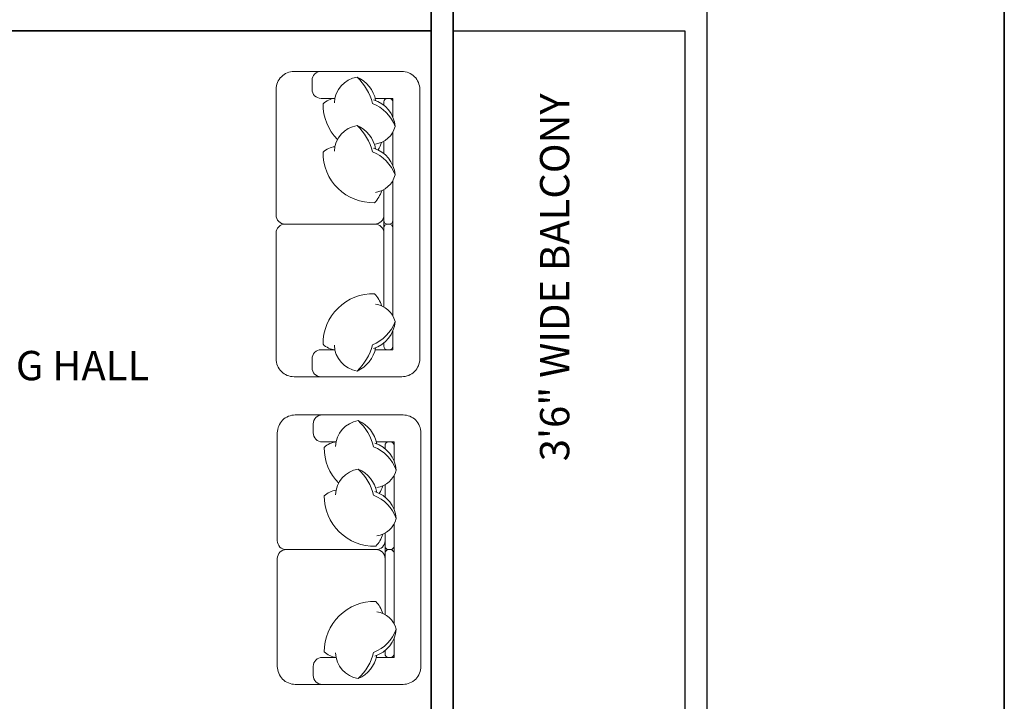
# Model space of a CAD drawing. Units: inches. Extents: x 1088 to 1703, y 668 to 1875.
# Tile 5 of 45: x 1502 to 1703, y 1189 to 1329. Entities that reach past the tile are written whole.
import ezdxf

# ---------------------------------------------------------------- set-up
doc = ezdxf.new("R2010")
doc.units = ezdxf.units.IN
for name, color, linetype, lineweight in [('A-ANNO-DIMS', 2, 'Continuous', 18), ('A-ANNO-TTLB', 7, 'Continuous', 35), ('A-AREA-IDEN', 7, 'Continuous', 18), ('A-FLOR-HRAL', 7, 'Continuous', 25), ('A-FURN', 8, 'Continuous', 13), ('A-WALL', 7, 'Continuous', 35)]:
    doc.layers.add(name, color=color, linetype=linetype, lineweight=lineweight)
doc.styles.get("Standard").update_dxf_attribs({"font": 'arial.ttf'})
doc.dimstyles.get("Standard").update_dxf_attribs({"dimtxt": 0.18, "dimasz": 0.18, "dimexe": 0.18, "dimexo": 0.0625, "dimgap": 0.09, "dimtad": 0, "dimtih": 1, "dimtoh": 1, "dimdec": 4, "dimzin": 0, "dimdsep": 46, "dimtxsty": 'Standard', "dimcen": 0.09, "dimadec": 0, "dimazin": 0, "dimtfac": 1, "dimtdec": 4, "dimtofl": 0, "dimtmove": 0, "dimatfit": 3, "dimfxl": 1, "dimtolj": 1, "dimtzin": 0, "dimarcsym": 0})

# ---------------------------------------------------------------- blocks, each defined once
blk = doc.blocks.new('*D31')
at = {"layer": 'A-ANNO-DIMS', "color": 0, "lineweight": -2, "transparency": 16777216}
for p, q in [((1435.84, 1326.5), (1435.84, 725.55)), ((1585.84, 1326.5), (1585.84, 725.55)), ((1436.02, 725.73), (1510.56, 725.73)), ((1585.66, 725.73), (1511.12, 725.73))]:
    blk.add_line(p, q, dxfattribs=at)
at = {"layer": 'A-ANNO-DIMS', "color": 0, "transparency": 16777216}
for points in [[(1436.02, 725.76), (1436.02, 725.7), (1435.84, 725.73)], [(1585.66, 725.76), (1585.66, 725.7), (1585.84, 725.73)]]:
    blk.add_solid(points, dxfattribs=at)
at = {"layer": 'Defpoints', "color": 0, "transparency": 16777216}
for p in [(1435.84, 1326.56), (1585.84, 1326.56), (1585.84, 725.73)]:
    blk.add_point(p, dxfattribs=at)
at = {"layer": 'A-ANNO-DIMS', "color": 0, "transparency": 16777216, "insert": (1510.84, 725.73), "char_height": 0.18, "attachment_point": 5}
blk.add_mtext('\\A1;150', dxfattribs=at)

msp = doc.modelspace()

# ---------------------------------------------------------------- linework, layer by layer
at = {"layer": 'A-ANNO-TTLB'}
msp.add_lwpolyline([(1088.369, 1874.677), (1703.181, 1874.677), (1703.181, 667.947), (1088.369, 667.947)], close=True, dxfattribs=at)
at = {"layer": 'A-FLOR-HRAL'}
for p, q in [((1642.243, 1331.058), (1642.243, 1181.058)), ((1590.345, 1326.558), (1637.743, 1326.558)), ((1637.743, 1326.558), (1637.743, 1185.558))]:
    msp.add_line(p, q, dxfattribs=at)
at = {"layer": 'A-FURN', "ltscale": 0.03}
for points in [[(1554.082, 1285.137, -0.4142136), (1555.92, 1286.975, -0.4142136), (1554.082, 1288.814), (1554.082, 1314.548, -0.4142136), (1557.759, 1318.225), (1579.817, 1318.225, -0.4142136), (1583.494, 1314.548), (1583.494, 1259.402, -0.4142136), (1579.817, 1255.726), (1557.759, 1255.726, -0.4142136), (1554.082, 1259.402), (1554.082, 1285.137, -0.4142136), (1555.92, 1286.975, -0.4142136), (1554.082, 1288.814)], [(1554.329, 1218.501, -0.4142136), (1556.167, 1220.339, -0.4142136), (1554.329, 1222.178), (1554.329, 1244.236, -0.4142136), (1558.006, 1247.912), (1580.064, 1247.912, -0.4142136), (1583.741, 1244.236), (1583.741, 1196.443, -0.4142136), (1580.064, 1192.766), (1558.006, 1192.766, -0.4142136), (1554.329, 1196.443), (1554.329, 1218.501, -0.4142136), (1556.167, 1220.339, -0.4142136), (1554.329, 1222.178)]]:
    msp.add_lwpolyline(points, format="xyb", dxfattribs=at)
at = {"layer": 'A-FURN'}
for points in [[(1566.121, 1312.71), (1563.273, 1312.71, -0.4142136), (1561.435, 1314.548), (1561.435, 1316.387, -0.4142136), (1563.273, 1318.225)], [(1566.01, 1311.788, -0.3567724), (1570.644, 1317.055, -0.2495421), (1574.462, 1312.282, 9.6168803)], [(1570.644, 1317.055, -0.1477299), (1573.803, 1311.682, -0.2133428), (1578.436, 1306.942, -0.1786618)], [(1566.122, 1312.714, 0.1655406), (1563.693, 1311.577, 0.2002311), (1566.651, 1304.28, 0.1215233)], [(1577.979, 1308.843), (1577.979, 1312.71), (1574.366, 1312.71, -0.4142136)], [(1576.141, 1311.307), (1576.141, 1311.975, -0.4142136), (1576.876, 1312.71), (1577.244, 1312.71, -0.4142136), (1577.979, 1311.975)], [(1574.054, 1312.425, -0.3066635), (1578.436, 1306.942, -0.30633), (1574.435, 1303.36, 0.8728472)], [(1577.979, 1311.975), (1577.979, 1308.843, -0.4142136)], [(1566.01, 1301.885, -0.3567724), (1570.644, 1307.153, -0.2495421), (1574.462, 1302.38, 9.6168803)], [(1570.644, 1307.153, -0.1477299), (1573.803, 1301.78, -0.2133428), (1578.436, 1297.04, -0.1786618)], [(1577.979, 1305.785), (1577.979, 1298.941, -0.4142136)], [(1566.122, 1302.812, 0.1655406), (1563.693, 1301.675, 0.4259892), (1574.224, 1291.351, 0.1215233), (1575.675, 1293.802, -7.1154643)], [(1574.054, 1302.522, -0.3066635), (1578.436, 1297.04, -0.30633), (1574.435, 1293.458, 0.8728472)], [(1574.957, 1302.163, 0.0718654), (1575.675, 1303.704, -7.1154643)], [(1576.141, 1301.405), (1576.141, 1303.934, -0.4142136)], [(1577.979, 1295.883), (1577.979, 1287.711, -0.4142136), (1577.244, 1286.975), (1576.876, 1286.975, -0.4142136), (1576.141, 1287.711), (1576.141, 1294.032, -0.4142136)], [(1576.141, 1288.814, -0.4142136), (1574.303, 1286.975), (1555.92, 1286.975, -0.4142136)], [(1576.141, 1288.814, -0.4142136), (1574.303, 1286.975)], [(1576.141, 1285.137, 0.4142136), (1574.303, 1286.975), (1555.92, 1286.975, 0.4142136)], [(1576.141, 1285.137, 0.4142136), (1574.303, 1286.975)], [(1577.979, 1268.166), (1577.979, 1286.24, 0.4142136), (1577.244, 1286.975), (1576.876, 1286.975, 0.4142136), (1576.141, 1286.24), (1576.141, 1270.017, 0.4142136)], [(1566.122, 1261.236, -0.1655406), (1563.693, 1262.374, -0.4259892), (1574.224, 1272.697, -0.1215233), (1575.675, 1270.247, 7.1154643)], [(1574.054, 1261.526, 0.3066635), (1578.436, 1267.009, 0.30633), (1574.435, 1270.59, -0.8728472)], [(1570.644, 1256.896, 0.1477299), (1573.803, 1262.268, 0.2133428), (1578.436, 1267.009, 0.1786618)], [(1577.979, 1261.976), (1577.979, 1265.108, 0.4142136)], [(1566.01, 1262.163, 0.3567724), (1570.644, 1256.896, 0.2495421), (1574.462, 1261.668, -9.6168803)], [(1576.141, 1262.643), (1576.141, 1261.976, 0.4142136), (1576.876, 1261.24), (1577.244, 1261.24, 0.4142136), (1577.979, 1261.976)], [(1563.273, 1255.726, -0.4142136), (1561.435, 1257.564), (1561.435, 1259.402, -0.4142136), (1563.273, 1261.24), (1566.121, 1261.24)], [(1566.368, 1242.398), (1563.52, 1242.398, -0.4142136), (1561.682, 1244.236), (1561.682, 1246.074, -0.4142136), (1563.52, 1247.912)], [(1566.257, 1241.475, -0.3567724), (1570.89, 1246.743, -0.2495421), (1574.709, 1241.97, 9.6168803)], [(1570.89, 1246.743, -0.1477299), (1574.05, 1241.37, -0.2133428), (1578.683, 1236.63, -0.1786618)], [(1566.369, 1242.402, 0.1655406), (1563.94, 1241.265, 0.2002311), (1566.898, 1233.968, 0.1215233)], [(1574.301, 1242.112, -0.3066635), (1578.683, 1236.63, -0.30633), (1574.681, 1233.048, 0.8728472)], [(1578.226, 1238.531), (1578.226, 1242.398), (1574.613, 1242.398, -0.4142136)], [(1576.388, 1240.995), (1576.388, 1241.663, -0.4142136), (1577.123, 1242.398), (1577.491, 1242.398, -0.4142136), (1578.226, 1241.663)], [(1578.226, 1241.663), (1578.226, 1238.531, -0.4142136)], [(1566.257, 1231.573, -0.3567724), (1570.89, 1236.84, -0.2495421), (1574.709, 1232.068, 9.6168803)], [(1570.89, 1236.84, -0.1477299), (1574.05, 1231.468, -0.2133428), (1578.683, 1226.727, -0.1786618)], [(1578.226, 1235.473), (1578.226, 1228.628, -0.4142136)], [(1566.369, 1232.5, 0.1655406), (1563.94, 1231.362, 0.4259892), (1574.471, 1221.039, 0.1215233), (1575.922, 1223.489, -7.1154643)], [(1574.301, 1232.21, -0.3066635), (1578.683, 1226.727, -0.30633), (1574.681, 1223.145, 0.8728472)], [(1575.204, 1231.85, 0.0718654), (1575.922, 1233.392, -7.1154643)], [(1576.388, 1231.093), (1576.388, 1233.622, -0.4142136)], [(1578.226, 1225.57), (1578.226, 1221.075, -0.4142136), (1577.491, 1220.339), (1577.123, 1220.339, -0.4142136), (1576.388, 1221.075), (1576.388, 1223.719, -0.4142136)], [(1576.388, 1222.178, -0.4142136), (1574.55, 1220.339), (1556.167, 1220.339, -0.4142136)], [(1576.388, 1222.178, -0.4142136), (1574.55, 1220.339)], [(1576.388, 1218.501, 0.4142136), (1574.55, 1220.339), (1556.167, 1220.339, 0.4142136)], [(1576.388, 1218.501, 0.4142136), (1574.55, 1220.339)], [(1578.226, 1205.206), (1578.226, 1219.604, 0.4142136), (1577.491, 1220.339), (1577.123, 1220.339, 0.4142136), (1576.388, 1219.604), (1576.388, 1207.057, 0.4142136)], [(1566.369, 1198.277, -0.1655406), (1563.94, 1199.414, -0.4259892), (1574.471, 1209.738, -0.1215233), (1575.922, 1207.287, 7.1154643)], [(1574.301, 1198.566, 0.3066635), (1578.683, 1204.049, 0.30633), (1574.681, 1207.631, -0.8728472)], [(1570.89, 1193.936, 0.1477299), (1574.05, 1199.309, 0.2133428), (1578.683, 1204.049, 0.1786618)], [(1578.226, 1199.016), (1578.226, 1202.148, 0.4142136)], [(1576.388, 1199.684), (1576.388, 1199.016, 0.4142136), (1577.123, 1198.281), (1577.491, 1198.281, 0.4142136), (1578.226, 1199.016)], [(1563.52, 1192.766, -0.4142136), (1561.682, 1194.604), (1561.682, 1196.443, -0.4142136), (1563.52, 1198.281), (1566.368, 1198.281)], [(1566.257, 1199.203, 0.3567724), (1570.89, 1193.936, 0.2495421), (1574.709, 1198.709, -9.6168803)]]:
    msp.add_lwpolyline(points, format="xyb", dxfattribs=at)
for points in [[(1577.979, 1298.941), (1577.979, 1305.785)], [(1577.979, 1268.166), (1577.979, 1295.883)], [(1574.366, 1261.24), (1577.979, 1261.24), (1577.979, 1265.108)], [(1578.226, 1228.628), (1578.226, 1235.473)], [(1578.226, 1205.206), (1578.226, 1225.57)], [(1574.613, 1198.281), (1578.226, 1198.281), (1578.226, 1202.148)]]:
    msp.add_lwpolyline(points, dxfattribs=at)
for points in [[(1577.979, 1286.24), (1577.979, 1287.711, -0.4142136), (1577.244, 1286.975), (1576.876, 1286.975, -0.4142136), (1576.141, 1287.711), (1576.141, 1286.24, -0.4142136), (1576.876, 1286.975), (1577.244, 1286.975, -0.4142136)], [(1578.226, 1219.604), (1578.226, 1221.075, -0.4142136), (1577.491, 1220.339), (1577.123, 1220.339, -0.4142136), (1576.388, 1221.075), (1576.388, 1219.604, -0.4142136), (1577.123, 1220.339), (1577.491, 1220.339, -0.4142136)]]:
    msp.add_lwpolyline(points, format="xyb", close=True, dxfattribs=at)
at = {"layer": 'A-WALL'}
for p, q in [((1585.845, 1415.058), (1585.845, 1185.558)), ((1590.345, 1415.058), (1590.345, 1185.558)), ((1435.845, 1326.558), (1585.845, 1326.558))]:
    msp.add_line(p, q, dxfattribs=at)

# ---------------------------------------------------------------- texts
at = {"layer": 'A-AREA-IDEN', "insert": (1608.113, 1238.429), "char_height": 6, "attachment_point": 1, "rotation": 90}
msp.add_mtext_dynamic_manual_height_columns('3\'6" WIDE BALCONY', width=128.79837, gutter_width=12.5, heights=[0], dxfattribs=at)
at = {"layer": 'A-AREA-IDEN', "insert": (1438.37, 1261.013), "char_height": 6, "attachment_point": 1}
msp.add_mtext_dynamic_manual_height_columns('DRAWING\\\\DINING HALL\\P13\'6"X21\'0"', width=91.5795, gutter_width=12.5, heights=[0], dxfattribs=at)

# ---------------------------------------------------------------- dimensions: what is measured, and where the dimension line sits
at = {"layer": 'A-ANNO-DIMS'}
dim = msp.add_linear_dim(base=(1585.845, 725.729), p1=(1435.845, 1326.558), p2=(1585.845, 1326.558), dimstyle='Standard', override={"dimdec": 0, "dimlfac": 1, "dimrnd": 0, "dimzin": 0, "dimdsep": 46, "dimlunit": 2}, dxfattribs=at)
dim.commit()
dim.dimension.update_dxf_attribs({"geometry": '*D31', "text_midpoint": (1510.845, 725.729)})

doc.saveas('drawing.dxf')
